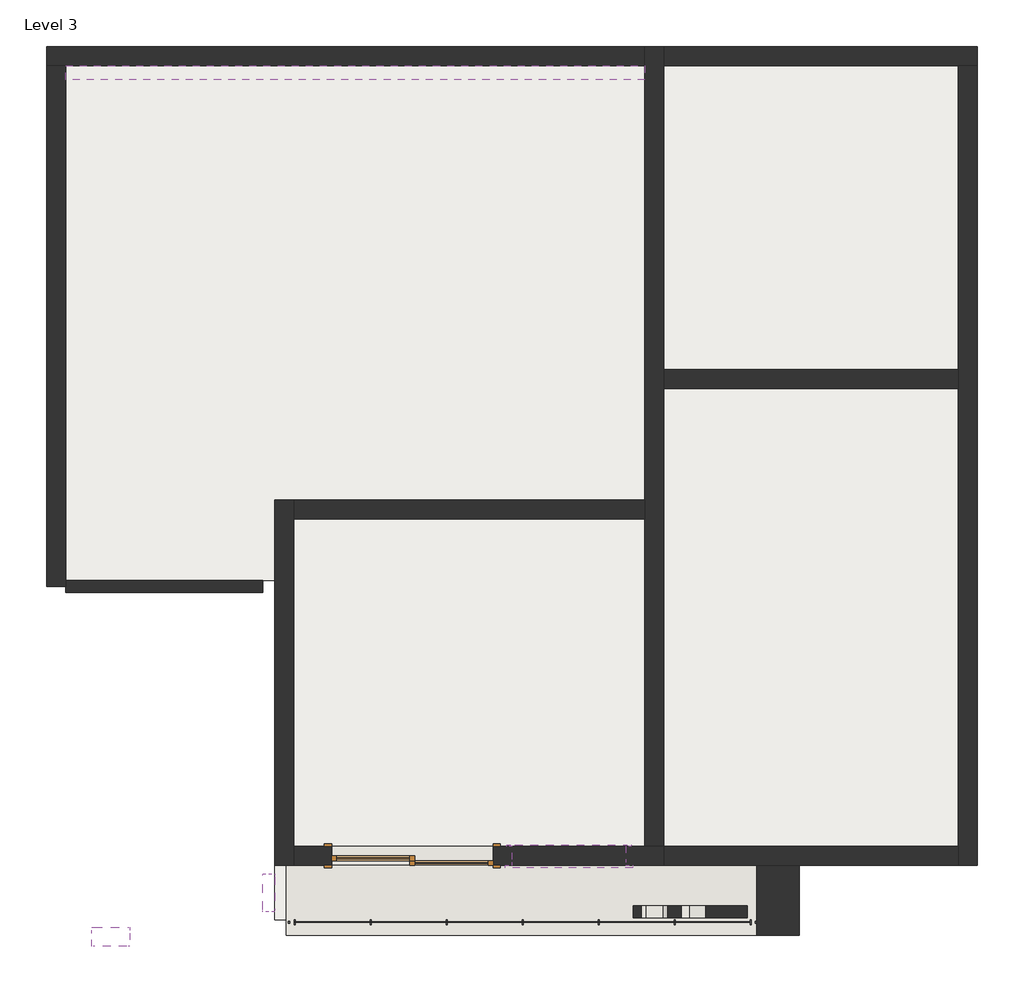
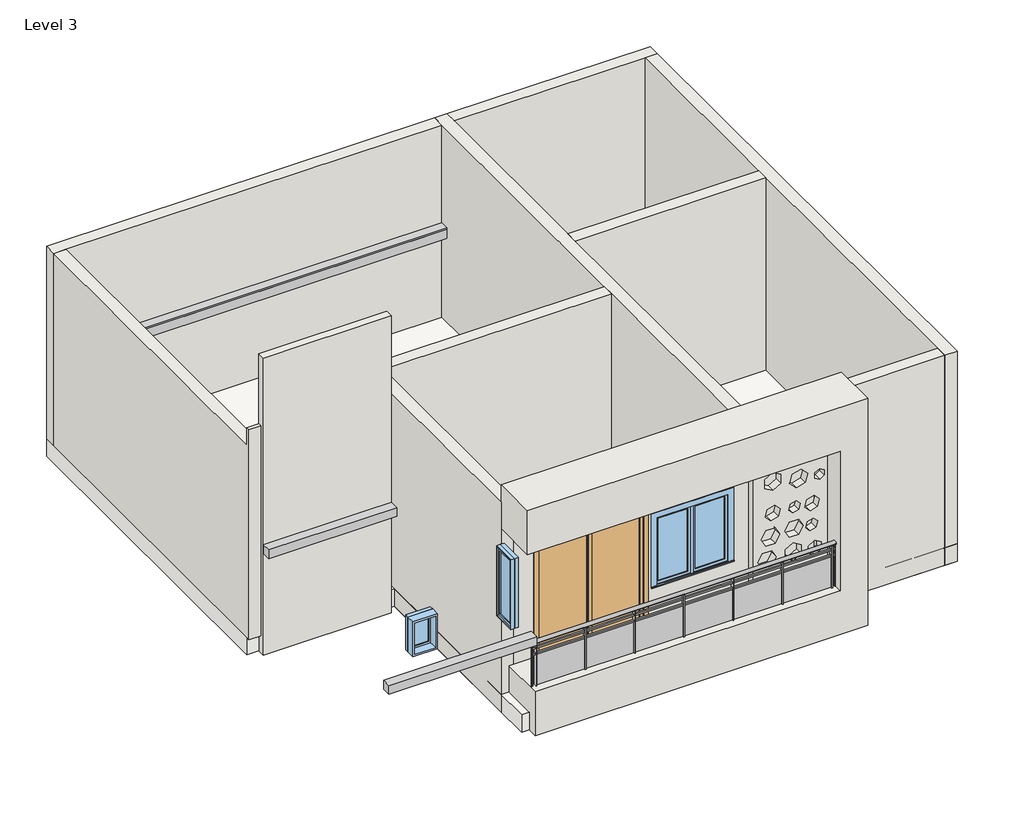
# One storey: 13 walls, 3 windows, 2 proxies, 1 door, 1 railing, 1 roof.
"""IFC4 building model written with IfcOpenShell, lengths in millimetres."""

from ifc_helpers import new_model, si_unit, point, frame, origin, place, context, project, spatial, polyline, ellipse_curve, trimmed, outline, extrude, faceted_brep, transform, mapped, element, save
from ifc_brep_helpers import plane_surface, extruded_surface, advanced_brep
from components import door_076b30e0, walls_1_walls_1_5292a9a1, window_0862ab64, window_085f26e1, window_f83fec05

model = new_model("IFC4")

# Units and contexts
model_context = context("Model", 3, world=origin())
ifc_project = project(units=[si_unit("LENGTHUNIT", "METRE", prefix="MILLI")], contexts=[model_context])

# Site, building, storey
site = spatial("IfcSite", under=ifc_project)
building = spatial("IfcBuilding", under=site)
storey = spatial("IfcBuildingStorey", under=building, Name="Level 3", Elevation=7315.2)

# Proxies
placement = place(None, origin())
element("IfcBuildingElementProxy", 1, Name="Cornice", ObjectType="Cornice", at=placement, inside=storey, context=model_context, shape_type="SweptSolid", body=[
    extrude(outline(polyline([(-5898.9432037, 9807.0548743), (-5898.9432037, 9654.6548743), (-12096.5432037, 9654.6548743), (-12096.5432037, 9807.0548743), (-5898.9432037, 9807.0548743)])), frame((0.0, 0.0, 9093.2), z_axis=(0.0, 0.0, 1.0), x_axis=(1.0, 0.0, 0.0)), (0.0, 0.0, 1.0), 152.4),
    extrude(outline(polyline([(-12299.7432037, 231.2548743), (-12299.7432037, 383.6548743), (-9861.3432037, 383.6548743), (-9861.3432037, 231.2548743), (-12299.7432037, 231.2548743)])), frame((0.0, 0.0, 9093.2), z_axis=(0.0, 0.0, 1.0), x_axis=(1.0, 0.0, 0.0)), (0.0, 0.0, 1.0), 152.4),
    extrude(outline(polyline([(-9988.3432037, 4168.2548743), (-9988.3432037, 4015.8548743), (-12096.5432037, 4015.8548743), (-12096.5432037, 4168.2548743), (-9988.3432037, 4168.2548743)])), frame((0.0, 0.0, 9093.2), z_axis=(0.0, 0.0, 1.0), x_axis=(1.0, 0.0, 0.0)), (0.0, 0.0, 1.0), 152.4),
])
element("IfcBuildingElementProxy", 2, Name="Cornice", ObjectType="Cornice", at=placement, inside=storey, context=model_context, shape_type="SweptSolid", body=[
    extrude(outline(polyline([(-5898.9432037, 9807.0548743), (-5898.9432037, 9654.6548743), (-12096.5432037, 9654.6548743), (-12096.5432037, 9807.0548743), (-5898.9432037, 9807.0548743)])), frame((0.0, 0.0, 9118.6), z_axis=(0.0, 0.0, 1.0), x_axis=(1.0, 0.0, 0.0)), (0.0, 0.0, 1.0), 152.4),
])

# Door
door_shape = door_076b30e0(model_context)
element("IfcDoor", 3, ObjectType="Door-Double-Sliding : 68\" x 80\"", at=placement, inside=storey, context=model_context, shape_type="MappedRepresentation", body=[
    mapped(door_shape, transform((-8388.1432037, 1475.8548743, 7924.8), x_axis=(-1.0, 0.0, 0.0), y_axis=(0.0, -1.0, 0.0), z_axis=(0.0, 0.0, 1.0))),
])

# Railing
element("IfcRailing", 4, ObjectType="Glass Panel - Bottom Fill", at=placement, inside=storey, context=model_context, shape_type="SolidModel", body=[
    advanced_brep(
    [(-9708.9432037, 675.7548743, 8839.2), (-9708.9432037, 599.5548743, 8839.2), (-4705.1432037, 675.7548743, 8839.2), (-4705.1432037, 599.5548743, 8839.2)],
    [
        (0, 1, ellipse_curve(frame((-9708.9432037, 637.6548743, 8839.2), z_axis=(-1.0, 0.0, 0.0), x_axis=(0.0, -1.0, 0.0)), 38.1, 28.575)),
        (1, 0, ellipse_curve(frame((-9708.9432037, 637.6548743, 8839.2), z_axis=(-1.0, 0.0, 0.0), x_axis=(0.0, -1.0, 0.0)), 38.1, 28.575)),
        (2, 3, ellipse_curve(frame((-4705.1432037, 637.6548743, 8839.2), z_axis=(1.0, 0.0, 0.0), x_axis=(0.0, -1.0, 0.0)), 38.1, 28.575)),
        (3, 2, ellipse_curve(frame((-4705.1432037, 637.6548743, 8839.2), z_axis=(1.0, 0.0, 0.0), x_axis=(0.0, -1.0, 0.0)), 38.1, 28.575)),
        (0, 2),
        (3, 1),
    ],
    [
        plane_surface(frame((-9708.9432037, 637.6548743, 8839.2), z_axis=(-1.0, 0.0, 0.0), x_axis=(0.0, 1.0, 0.0))),
        plane_surface(frame((-4705.1432037, 637.6548743, 8839.2), z_axis=(1.0, 0.0, 0.0), x_axis=(0.0, 1.0, 0.0))),
        extruded_surface(trimmed(ellipse_curve(frame((-4705.1432037, 637.6548743, 8839.2), z_axis=(-1.0, 0.0, 0.0), x_axis=(0.0, -1.0, 0.0)), 38.1, 28.575), [point((-4705.1432037, 675.7548743, 8839.2))], [point((-4705.1432037, 599.5548743, 8839.2))], True, "CARTESIAN"), (-5003.8, 0.0, 0.0), 5003.8),
        extruded_surface(trimmed(ellipse_curve(frame((-4705.1432037, 637.6548743, 8839.2), z_axis=(-1.0, 0.0, 0.0), x_axis=(0.0, -1.0, 0.0)), 38.1, 28.575), [point((-4705.1432037, 599.5548743, 8839.2))], [point((-4705.1432037, 675.7548743, 8839.2))], True, "CARTESIAN"), (-5003.8, 0.0, 0.0), 5003.8),
    ],
    [
        (0, [[1, 2]]),
        (1, [[3, 4]]),
        (2, [[-1, 5, -4, 6]]),
        (3, [[-2, -6, -3, -5]]),
    ],
),
    extrude(outline(polyline([(-9708.9432037, 624.9548743), (-9708.9432037, 650.3548743), (-4705.1432037, 650.3548743), (-4705.1432037, 624.9548743), (-9708.9432037, 624.9548743)])), frame((0.0, 0.0, 8724.9), z_axis=(0.0, 0.0, 1.0), x_axis=(1.0, 0.0, 0.0)), (0.0, 0.0, 1.0), 25.4),
    extrude(outline(polyline([(-9708.9432037, 624.9548743), (-9708.9432037, 650.3548743), (-4705.1432037, 650.3548743), (-4705.1432037, 624.9548743), (-9708.9432037, 624.9548743)])), frame((0.0, 0.0, 8623.3), z_axis=(0.0, 0.0, 1.0), x_axis=(1.0, 0.0, 0.0)), (0.0, 0.0, 1.0), 25.4),
    extrude(outline(polyline([(-4774.9932037, 612.2548743), (-4774.9932037, 663.0548743), (-4762.2932037, 663.0548743), (-4762.2932037, 612.2548743), (-4774.9932037, 612.2548743)])), frame((0.0, 0.0, 7924.8), z_axis=(0.0, 0.0, 1.0), x_axis=(1.0, 0.0, 0.0)), (0.0, 0.0, 1.0), 885.6788223),
    extrude(outline(polyline([(-5581.4432037, 644.1900313), (-4768.6432037, 644.1900313), (-4768.6432037, 637.8400313), (-5581.4432037, 637.8400313), (-5581.4432037, 644.1900313)])), frame((0.0, 0.0, 8026.4), z_axis=(0.0, 0.0, 1.0), x_axis=(1.0, 0.0, 0.0)), (0.0, 0.0, 1.0), 596.9),
    extrude(outline(polyline([(-5587.7932037, 612.2548743), (-5587.7932037, 663.0548743), (-5575.0932037, 663.0548743), (-5575.0932037, 612.2548743), (-5587.7932037, 612.2548743)])), frame((0.0, 0.0, 7924.8), z_axis=(0.0, 0.0, 1.0), x_axis=(1.0, 0.0, 0.0)), (0.0, 0.0, 1.0), 885.6788223),
    extrude(outline(polyline([(-6394.2432037, 644.1900313), (-5581.4432037, 644.1900313), (-5581.4432037, 637.8400313), (-6394.2432037, 637.8400313), (-6394.2432037, 644.1900313)])), frame((0.0, 0.0, 8026.4), z_axis=(0.0, 0.0, 1.0), x_axis=(1.0, 0.0, 0.0)), (0.0, 0.0, 1.0), 596.9),
    extrude(outline(polyline([(-6400.5932037, 612.2548743), (-6400.5932037, 663.0548743), (-6387.8932037, 663.0548743), (-6387.8932037, 612.2548743), (-6400.5932037, 612.2548743)])), frame((0.0, 0.0, 7924.8), z_axis=(0.0, 0.0, 1.0), x_axis=(1.0, 0.0, 0.0)), (0.0, 0.0, 1.0), 885.6788223),
    extrude(outline(polyline([(-7207.0432037, 644.1900313), (-6394.2432037, 644.1900313), (-6394.2432037, 637.8400313), (-7207.0432037, 637.8400313), (-7207.0432037, 644.1900313)])), frame((0.0, 0.0, 8026.4), z_axis=(0.0, 0.0, 1.0), x_axis=(1.0, 0.0, 0.0)), (0.0, 0.0, 1.0), 596.9),
    extrude(outline(polyline([(-7213.3932037, 612.2548743), (-7213.3932037, 663.0548743), (-7200.6932037, 663.0548743), (-7200.6932037, 612.2548743), (-7213.3932037, 612.2548743)])), frame((0.0, 0.0, 7924.8), z_axis=(0.0, 0.0, 1.0), x_axis=(1.0, 0.0, 0.0)), (0.0, 0.0, 1.0), 885.6788223),
    extrude(outline(polyline([(-8019.8432037, 644.1900313), (-7207.0432037, 644.1900313), (-7207.0432037, 637.8400313), (-8019.8432037, 637.8400313), (-8019.8432037, 644.1900313)])), frame((0.0, 0.0, 8026.4), z_axis=(0.0, 0.0, 1.0), x_axis=(1.0, 0.0, 0.0)), (0.0, 0.0, 1.0), 596.9),
    extrude(outline(polyline([(-8026.1932037, 612.2548743), (-8026.1932037, 663.0548743), (-8013.4932037, 663.0548743), (-8013.4932037, 612.2548743), (-8026.1932037, 612.2548743)])), frame((0.0, 0.0, 7924.8), z_axis=(0.0, 0.0, 1.0), x_axis=(1.0, 0.0, 0.0)), (0.0, 0.0, 1.0), 885.6788223),
    extrude(outline(polyline([(-8832.6432037, 644.1900313), (-8019.8432037, 644.1900313), (-8019.8432037, 637.8400313), (-8832.6432037, 637.8400313), (-8832.6432037, 644.1900313)])), frame((0.0, 0.0, 8026.4), z_axis=(0.0, 0.0, 1.0), x_axis=(1.0, 0.0, 0.0)), (0.0, 0.0, 1.0), 596.9),
    extrude(outline(polyline([(-8838.9932037, 612.2548743), (-8838.9932037, 663.0548743), (-8826.2932037, 663.0548743), (-8826.2932037, 612.2548743), (-8838.9932037, 612.2548743)])), frame((0.0, 0.0, 7924.8), z_axis=(0.0, 0.0, 1.0), x_axis=(1.0, 0.0, 0.0)), (0.0, 0.0, 1.0), 885.6788223),
    extrude(outline(polyline([(-9645.4432037, 644.1900313), (-8832.6432037, 644.1900313), (-8832.6432037, 637.8400313), (-9645.4432037, 637.8400313), (-9645.4432037, 644.1900313)])), frame((0.0, 0.0, 8026.4), z_axis=(0.0, 0.0, 1.0), x_axis=(1.0, 0.0, 0.0)), (0.0, 0.0, 1.0), 596.9),
    extrude(outline(polyline([(-9651.7932037, 612.2548743), (-9651.7932037, 663.0548743), (-9639.0932037, 663.0548743), (-9639.0932037, 612.2548743), (-9651.7932037, 612.2548743)])), frame((0.0, 0.0, 7924.8), z_axis=(0.0, 0.0, 1.0), x_axis=(1.0, 0.0, 0.0)), (0.0, 0.0, 1.0), 885.6788223),
    extrude(outline(polyline([(-4717.8432037, 628.1298743), (-4717.8432037, 647.1798743), (-4698.7932037, 647.1798743), (-4698.7932037, 628.1298743), (-4717.8432037, 628.1298743)])), frame((0.0, 0.0, 7924.8), z_axis=(0.0, 0.0, 1.0), x_axis=(1.0, 0.0, 0.0)), (0.0, 0.0, 1.0), 885.6788223),
    extrude(outline(polyline([(-9715.2932037, 628.1298743), (-9715.2932037, 647.1798743), (-9696.2432037, 647.1798743), (-9696.2432037, 628.1298743), (-9715.2932037, 628.1298743)])), frame((0.0, 0.0, 7924.8), z_axis=(0.0, 0.0, 1.0), x_axis=(1.0, 0.0, 0.0)), (0.0, 0.0, 1.0), 885.6788223),
])

# Roof
element("IfcRoof", 5, ObjectType="Generic - 12\"", at=placement, inside=storey, context=model_context, shape_type="SweptSolid", body=[
    extrude(outline(polyline([(-12299.7432037, 10010.2548743), (-2342.9432037, 10010.2548743), (-2342.9432037, 1247.2548743), (-4247.9432037, 1247.2548743), (-4247.9432037, 663.0548743), (-9861.3432037, 663.0548743), (-9861.3432037, 1298.0548743), (-9861.3432037, 4295.2548743), (-12299.7432037, 4295.2548743), (-12299.7432037, 10010.2548743)])), frame((0.0, 0.0, 7315.2), z_axis=(0.0, 0.0, 1.0), x_axis=(1.0, 0.0, 0.0)), (0.0, 0.0, 1.0), 304.8),
])

# Walls
element("IfcWall", 6, ObjectType="Generic - 5\"", at=placement, inside=storey, context=model_context, shape_type="Brep", body=[
    faceted_brep([(-9988.3432037, 4295.2548743, 7315.2), (-12096.5432037, 4295.2548743, 7315.2), (-12096.5432037, 4295.2548743, 7620.0), (-12096.5432037, 4295.2548743, 10972.8), (-12096.5432037, 4295.2548743, 11277.6), (-12096.5432037, 4295.2548743, 12496.8), (-9988.3432037, 4295.2548743, 12496.8), (-9988.3432037, 4168.2548743, 7315.2), (-9988.3432037, 4168.2548743, 12496.8), (-12096.5432037, 4168.2548743, 12496.8), (-12096.5432037, 4168.2548743, 7315.2), (-12096.5432037, 4231.7548743, 7315.2)], [[[0, 1, 2, 3, 4, 5, 6]], [[7, 8, 9, 10]], [[1, 0, 7, 10, 11]], [[6, 5, 9, 8]], [[0, 6, 8, 7]], [[1, 11, 10, 9, 5, 4, 3, 2]]]),
])
element("IfcWall", 7, ObjectType="Generic - 5\"", at=placement, inside=storey, context=model_context, shape_type="SweptSolid", body=[
    extrude(outline(polyline([(8068.6361055, -4806.7432037), (10508.7650496, -4806.7432037), (10508.7650496, -6025.9432037), (8068.6361055, -6025.9432037), (8068.6361055, -4806.7432037)]), holes=[polyline([(10140.6755343, -5569.437477), (10064.4755343, -5701.4197485), (10140.6755343, -5833.4020201), (10293.0755343, -5833.4020201), (10369.2755343, -5701.4197485), (10293.0755343, -5569.437477), (10140.6755343, -5569.437477)]), polyline([(10163.9613965, -5130.2790834), (10016.7543006, -5169.7231059), (9977.3102781, -5316.9302018), (10085.0733516, -5424.6932753), (10232.2804475, -5385.2492528), (10271.72447, -5238.0421569), (10163.9613965, -5130.2790834)]), polyline([(9703.2041949, -5578.7471686), (9580.531615, -5611.6171873), (9547.6615962, -5734.2897672), (9637.4641574, -5824.0923285), (9760.1367374, -5791.2223097), (9793.0067561, -5668.5497298), (9703.2041949, -5578.7471686)]), polyline([(9678.1574319, -5247.2726782), (9580.019368, -5273.5686932), (9553.723353, -5371.7067571), (9625.565402, -5443.5488061), (9723.7034659, -5417.2527911), (9749.9994809, -5319.1147272), (9678.1574319, -5247.2726782)]), polyline([(9264.0488124, -5590.7002981), (9132.0665409, -5666.9002981), (9132.0665409, -5819.3002981), (9264.0488124, -5895.5002981), (9396.0310839, -5819.3002981), (9396.0310839, -5666.9002981), (9264.0488124, -5590.7002981)]), polyline([(9279.67242, -5201.6464153), (9147.6901485, -5277.8464153), (9147.6901485, -5430.2464153), (9279.67242, -5506.4464153), (9411.6546915, -5430.2464153), (9411.6546915, -5277.8464153), (9279.67242, -5201.6464153)]), polyline([(9272.6391638, -4966.188489), (9174.5010999, -4992.484504), (9148.2050849, -5090.6225679), (9220.0471339, -5162.4646169), (9318.1851978, -5136.1686019), (9344.4812128, -5038.030538), (9272.6391638, -4966.188489)]), polyline([(9646.9071324, -4934.22274), (9524.2345525, -4967.0927588), (9491.3645338, -5089.7653387), (9581.167095, -5179.5678999), (9703.8396749, -5146.6978812), (9736.7096937, -5024.0253012), (9646.9071324, -4934.22274)]), polyline([(10035.431483, -4853.8956856), (9990.3878062, -4931.9136222), (10035.431483, -5009.9315589), (10125.5188364, -5009.9315589), (10170.5625131, -4931.9136222), (10125.5188364, -4853.8956856), (10035.431483, -4853.8956856)]), polyline([(8887.3926853, -5644.9432037), (8755.4104138, -5721.1432037), (8755.4104138, -5873.5432037), (8887.3926853, -5949.7432037), (9019.3749569, -5873.5432037), (9019.3749569, -5721.1432037), (8887.3926853, -5644.9432037)]), polyline([(8801.9964308, -5235.9460501), (8725.7964308, -5367.9283217), (8801.9964308, -5499.9105932), (8954.3964308, -5499.9105932), (9030.5964308, -5367.9283217), (8954.3964308, -5235.9460501), (8801.9964308, -5235.9460501)]), polyline([(8761.231321, -4901.3742658), (8697.731321, -5011.3594921), (8761.231321, -5121.3447183), (8888.231321, -5121.3447183), (8951.731321, -5011.3594921), (8888.231321, -4901.3742658), (8761.231321, -4901.3742658)]), polyline([(8450.6104138, -5618.3643314), (8295.6101636, -5707.8537676), (8295.6101636, -5886.8326399), (8450.6104138, -5976.3220761), (8605.610664, -5886.8326399), (8605.610664, -5707.8537676), (8450.6104138, -5618.3643314)]), polyline([(8468.3460703, -5203.5482833), (8295.6101636, -5249.83273), (8249.3257169, -5422.5686367), (8375.7771769, -5549.0200966), (8548.5130835, -5502.7356499), (8594.7975302, -5329.9997433), (8468.3460703, -5203.5482833)]), polyline([(8389.7874753, -4898.3582178), (8278.2141342, -4928.2542045), (8248.3181476, -5039.8275455), (8329.995502, -5121.5048999), (8441.5688431, -5091.6089133), (8471.4648297, -4980.0355722), (8389.7874753, -4898.3582178)])]), frame((0.0, 688.4548476, 0.0), z_axis=(0.0, 1.0, 0.0), x_axis=(0.0, 0.0, 1.0)), (0.0, 0.0, 1.0), 127.0),
])
element("IfcWall", 8, ObjectType="Generic - 8\"", at=placement, inside=storey, context=model_context, shape_type="Brep", body=[
    faceted_brep([(-9861.3432037, 5158.8548743, 7315.2), (-9861.3432037, 1247.2548743, 7315.2), (-9861.3432037, 1247.2548743, 10972.8), (-9861.3432037, 1298.0548743, 10972.8), (-9861.3432037, 4295.2548743, 10972.8), (-9861.3432037, 5158.8548743, 10972.8), (-9658.1432037, 5158.8548743, 7315.2), (-9658.1432037, 5158.8548743, 10972.8), (-9658.1432037, 4955.6548743, 10972.8), (-9658.1432037, 1450.4548743, 10972.8), (-9658.1432037, 1247.2548743, 10972.8), (-9658.1432037, 1247.2548743, 7315.2), (-9658.1432037, 1450.4548743, 7315.2), (-9658.1432037, 4955.6548743, 7315.2)], [[[0, 1, 2, 3, 4, 5]], [[6, 7, 8, 9, 10, 11, 12, 13]], [[1, 0, 6, 13, 12, 11]], [[2, 1, 11, 10]], [[0, 5, 7, 6]], [[5, 4, 3, 2, 10, 9, 8, 7]]]),
])
element("IfcWall", 9, ObjectType="Generic - 8\"", at=placement, inside=storey, context=model_context, shape_type="Brep", body=[
    faceted_brep([(-9658.1432037, 1247.2548743, 7315.2), (-5695.7432037, 1247.2548743, 7315.2), (-5695.7432037, 1247.2548743, 10972.8), (-9658.1432037, 1247.2548743, 10972.8), (-7524.5432037, 1247.2548743, 9956.8), (-7524.5432037, 1247.2548743, 7924.8), (-9251.7432037, 1247.2548743, 7924.8), (-9251.7432037, 1247.2548743, 9956.8), (-7321.3432037, 1247.2548743, 9833.9107901), (-6102.1432037, 1247.2548743, 9833.9107901), (-6102.1432037, 1247.2548743, 8614.7107901), (-7321.3432037, 1247.2548743, 8614.7107901), (-9658.1432037, 1450.4548743, 7315.2), (-9658.1432037, 1450.4548743, 10972.8), (-5898.9432037, 1450.4548743, 10972.8), (-5695.7432037, 1450.4548743, 10972.8), (-5695.7432037, 1450.4548743, 7315.2), (-5898.9432037, 1450.4548743, 7315.2), (-7524.5432037, 1450.4548743, 9956.8), (-9251.7432037, 1450.4548743, 9956.8), (-9251.7432037, 1450.4548743, 7924.8), (-7524.5432037, 1450.4548743, 7924.8), (-7321.3432037, 1450.4548743, 9833.9107901), (-7321.3432037, 1450.4548743, 8614.7107901), (-6102.1432037, 1450.4548743, 8614.7107901), (-6102.1432037, 1450.4548743, 9833.9107901)], [[[0, 1, 2, 3], [4, 5, 6, 7], [8, 9, 10, 11]], [[12, 13, 14, 15, 16, 17], [18, 19, 20, 21], [22, 23, 24, 25]], [[1, 0, 12, 17, 16]], [[0, 3, 13, 12]], [[2, 1, 16, 15]], [[3, 2, 15, 14, 13]], [[5, 4, 18, 21]], [[6, 5, 21, 20]], [[7, 6, 20, 19]], [[4, 7, 19, 18]], [[23, 22, 8, 11]], [[24, 23, 11, 10]], [[25, 24, 10, 9]], [[22, 25, 9, 8]]]),
])
element("IfcWall", 10, ObjectType="Generic - 8\"", at=placement, inside=storey, context=model_context, shape_type="Brep", body=[
    faceted_brep([(-5695.7432037, 1450.4548743, 7315.2), (-5695.7432037, 6352.6548743, 7315.2), (-5695.7432037, 6555.8548743, 7315.2), (-5695.7432037, 9807.0548743, 7315.2), (-5695.7432037, 10010.2548743, 7315.2), (-5695.7432037, 10010.2548743, 10972.8), (-5695.7432037, 9807.0548743, 10972.8), (-5695.7432037, 6555.8548743, 10972.8), (-5695.7432037, 6352.6548743, 10972.8), (-5695.7432037, 5362.0548743, 10972.8), (-5695.7432037, 1450.4548743, 10972.8), (-5898.9432037, 1450.4548743, 7315.2), (-5898.9432037, 1450.4548743, 10972.8), (-5898.9432037, 4955.6548743, 10972.8), (-5898.9432037, 5158.8548743, 10972.8), (-5898.9432037, 5362.0548743, 10972.8), (-5898.9432037, 9807.0548743, 10972.8), (-5898.9432037, 10010.2548743, 10972.8), (-5898.9432037, 10010.2548743, 7620.0), (-5898.9432037, 10010.2548743, 7315.2), (-5898.9432037, 5158.8548743, 7315.2), (-5898.9432037, 4955.6548743, 7315.2)], [[[0, 1, 2, 3, 4, 5, 6, 7, 8, 9, 10]], [[11, 12, 13, 14, 15, 16, 17, 18, 19, 20, 21]], [[4, 3, 2, 1, 0, 11, 21, 20, 19]], [[0, 10, 12, 11]], [[10, 9, 8, 7, 6, 5, 17, 16, 15, 14, 13, 12]], [[4, 19, 18, 17, 5]]]),
])
element("IfcWall", 11, ObjectType="Generic - 8\"", at=placement, inside=storey, context=model_context, shape_type="SweptSolid", body=[
    extrude(outline(polyline([(-2546.1432037, 6352.6548743), (-5695.7432037, 6352.6548743), (-5695.7432037, 6555.8548743), (-2546.1432037, 6555.8548743), (-2546.1432037, 6352.6548743)])), frame((0.0, 0.0, 7315.2), z_axis=(0.0, 0.0, 1.0), x_axis=(1.0, 0.0, 0.0)), (0.0, 0.0, 1.0), 3657.6),
])
element("IfcWall", 12, ObjectType="Generic - 8\"", at=placement, inside=storey, context=model_context, shape_type="Brep", body=[
    faceted_brep([(-2546.1432037, 9807.0548743, 7315.2), (-2546.1432037, 6555.8548743, 7315.2), (-2546.1432037, 6352.6548743, 7315.2), (-2546.1432037, 1450.4548743, 7315.2), (-2546.1432037, 1247.2548743, 7315.2), (-2546.1432037, 1247.2548743, 10972.8), (-2546.1432037, 1450.4548743, 10972.8), (-2546.1432037, 6352.6548743, 10972.8), (-2546.1432037, 6555.8548743, 10972.8), (-2546.1432037, 9807.0548743, 10972.8), (-2342.9432037, 9807.0548743, 7315.2), (-2342.9432037, 9807.0548743, 10972.8), (-2342.9432037, 1247.2548743, 10972.8), (-2342.9432037, 1247.2548743, 7315.2)], [[[0, 1, 2, 3, 4, 5, 6, 7, 8, 9]], [[10, 11, 12, 13]], [[4, 3, 2, 1, 0, 10, 13]], [[5, 4, 13, 12]], [[0, 9, 11, 10]], [[9, 8, 7, 6, 5, 12, 11]]]),
])
element("IfcWall", 13, ObjectType="Generic - 8\"", at=placement, inside=storey, context=model_context, shape_type="Brep", body=[
    faceted_brep([(-5695.7432037, 1247.2548743, 7315.2), (-2546.1432037, 1247.2548743, 7315.2), (-2546.1432037, 1247.2548743, 10972.8), (-4247.9432037, 1247.2548743, 10972.8), (-5695.7432037, 1247.2548743, 10972.8), (-5695.7432037, 1450.4548743, 7315.2), (-5695.7432037, 1450.4548743, 10972.8), (-2546.1432037, 1450.4548743, 10972.8), (-2546.1432037, 1450.4548743, 7315.2)], [[[0, 1, 2, 3, 4]], [[5, 6, 7, 8]], [[1, 0, 5, 8]], [[0, 4, 6, 5]], [[2, 1, 8, 7]], [[4, 3, 2, 7, 6]]]),
])
element("IfcWall", 14, ObjectType="Generic - 8\"", at=placement, inside=storey, context=model_context, shape_type="SweptSolid", body=[
    extrude(outline(polyline([(-5898.9432037, 4955.6548743), (-9658.1432037, 4955.6548743), (-9658.1432037, 5158.8548743), (-5898.9432037, 5158.8548743), (-5898.9432037, 4955.6548743)])), frame((0.0, 0.0, 7315.2), z_axis=(0.0, 0.0, 1.0), x_axis=(1.0, 0.0, 0.0)), (0.0, 0.0, 1.0), 3657.6),
])
element("IfcWall", 15, ObjectType="Generic - 8\"", at=placement, inside=storey, context=model_context, shape_type="Brep", body=[
    faceted_brep([(-5695.7432037, 9807.0548743, 10972.8), (-5695.7432037, 9807.0548743, 7315.2), (-2546.1432037, 9807.0548743, 7315.2), (-2342.9432037, 9807.0548743, 7315.2), (-2342.9432037, 9807.0548743, 10972.8), (-2546.1432037, 9807.0548743, 10972.8), (-5695.7432037, 10010.2548743, 7315.2), (-5695.7432037, 10010.2548743, 10972.8), (-2342.9432037, 10010.2548743, 10972.8), (-2342.9432037, 10010.2548743, 7315.2), (-5695.7432037, 9832.4548743, 10972.8)], [[[0, 1, 2, 3, 4, 5]], [[6, 7, 8, 9]], [[3, 2, 1, 6, 9]], [[4, 3, 9, 8]], [[0, 5, 4, 8, 7, 10]], [[0, 10, 7, 6, 1]]]),
])
element("IfcWall", 16, ObjectType="Generic - 8\"", at=placement, inside=storey, context=model_context, shape_type="Brep", body=[
    faceted_brep([(-5898.9432037, 10010.2548743, 10972.8), (-5898.9432037, 10010.2548743, 7620.0), (-12299.7432037, 10010.2548743, 7620.0), (-12299.7432037, 10010.2548743, 10972.8), (-5898.9432037, 9807.0548743, 7620.0), (-5898.9432037, 9807.0548743, 10972.8), (-12096.5432037, 9807.0548743, 10972.8), (-12299.7432037, 9807.0548743, 10972.8), (-12299.7432037, 9807.0548743, 7620.0), (-12096.5432037, 9807.0548743, 7620.0)], [[[0, 1, 2, 3]], [[4, 5, 6, 7, 8, 9]], [[2, 1, 4, 9, 8]], [[3, 2, 8, 7]], [[0, 3, 7, 6, 5]], [[0, 5, 4, 1]]]),
])
element("IfcWall", 17, ObjectType="Generic - 8\"", at=placement, inside=storey, context=model_context, shape_type="Brep", body=[
    faceted_brep([(-12299.7432037, 9807.0548743, 7620.0), (-12299.7432037, 4295.2548743, 7620.0), (-12299.7432037, 4231.7548743, 7620.0), (-12299.7432037, 4231.7548743, 11277.6), (-12299.7432037, 4295.2548743, 11277.6), (-12299.7432037, 4295.2548743, 10972.8), (-12299.7432037, 9807.0548743, 10972.8), (-12096.5432037, 4231.7548743, 7620.0), (-12096.5432037, 4295.2548743, 7620.0), (-12096.5432037, 9807.0548743, 7620.0), (-12096.5432037, 9807.0548743, 9093.2), (-12096.5432037, 9807.0548743, 9245.6), (-12096.5432037, 9807.0548743, 10972.8), (-12096.5432037, 4295.2548743, 10972.8), (-12096.5432037, 4295.2548743, 11277.6), (-12096.5432037, 4231.7548743, 11277.6)], [[[0, 1, 2, 3, 4, 5, 6]], [[7, 8, 9, 10, 11, 12, 13, 14, 15]], [[2, 1, 0, 9, 8, 7]], [[3, 2, 7, 15]], [[0, 6, 12, 11, 10, 9]], [[3, 15, 14, 4]], [[12, 6, 5, 13]], [[4, 14, 13, 5]]]),
])
walls_1_walls_1_shape = walls_1_walls_1_5292a9a1(model_context)
element("IfcWall", 18, ObjectType="Walls 1 : Walls 1", at=placement, inside=storey, context=model_context, shape_type="MappedRepresentation", body=[
    mapped(walls_1_walls_1_shape, transform((0.0, 0.0, 0.0), x_axis=(1.0, 0.0, 0.0), y_axis=(0.0, 1.0, 0.0), z_axis=(0.0, 0.0, 1.0))),
])

# Windows
window_shape = window_0862ab64(model_context)
element("IfcWindow", 19, ObjectType="Casement Dbl with Trim : 48\" x 48\"", at=placement, inside=storey, context=model_context, shape_type="MappedRepresentation", body=[
    mapped(window_shape, transform((-6711.7432037, 1367.9048743, 7700.3107901), x_axis=(-1.0, 0.0, 0.0), y_axis=(0.0, -1.0, 0.0), z_axis=(0.0, 0.0, 1.0))),
])
window_2_shape = window_085f26e1(model_context)
element("IfcWindow", 20, ObjectType="Fixed : 16\" x 24\"", at=placement, inside=storey, context=model_context, shape_type="MappedRepresentation", body=[
    mapped(window_2_shape, transform((-11575.8432037, 485.2548743, 8571.2555904), x_axis=(1.0, 0.0, 0.0), y_axis=(0.0, 1.0, 0.0), z_axis=(0.0, 0.0, 1.0))),
])
window_3_shape = window_f83fec05(model_context)
element("IfcWindow", 21, ObjectType="Fixed : 16\" x 48\"", at=placement, inside=storey, context=model_context, shape_type="MappedRepresentation", body=[
    mapped(window_3_shape, transform((-9924.8432037, 993.2548743, 8180.6841054), x_axis=(0.0, 1.0, 0.0), y_axis=(-1.0, 0.0, 0.0), z_axis=(0.0, 0.0, 1.0))),
])

save(model, "model.ifc")

# Revit data of these elements
# Type "Door-Double-Sliding : 68\" x 80\""
#   Type Mark = "8"
#   Construction Type Id = "opn-d45"
#   Assembly Code = "C1020"
#   Analytic Construction = "Wood frame, double glass door "
#   Thickness = 0' - 2"
#   Thermal Resistance (R) = 1.8150 (h·ft²·°F)/BTU
#   Heat Transfer Coefficient (U) = 0.5510 BTU/(h·ft²·°F)
#   Height = 6' - 8"
#   Rail Width = 0' - 2"
#   Stiles = 0' - 2"
#   Trim Projection Ext = 0' - 1"
#   Trim Projection Int = 0' - 1"
#   Trim Width = 0' - 3"
#   Width = 5' - 8"
#   Define Thermal Properties by = 1
#   Glazing = Glass
#   Panel Material = Wood - Birch - Solid Stained Light Low Gloss
#   Trim Material = Paint - Sienna
#   Visual Light Transmittance = 0
#   Solar Heat Gain Coefficient = 0
#   Function = (empty or 0)
#   Wall Closure = (empty or 0)
# Type "Glass Panel - Bottom Fill"
#   Assembly Code = "C2010400"
#   built-in parameter 1008612 = 0.0416667 (stored number, unit not read)
#   built-in parameter 1008611 = 0.0416667 (stored number, unit not read)
#   built-in parameter 1008609 = 0.333333 (stored number, unit not read)
#   built-in parameter 1008604 = 0.166667 (stored number, unit not read)
#   built-in parameter 1008603 = 0.166667 (stored number, unit not read)
#   Railing Height = 3' - 0"
#   built-in parameter 1008630 = 2
#   built-in parameter 1008610 = 2
#   built-in parameter 1008618 = Baluster - Square : 3/4"
# Type "Generic - 12\""
#   Assembly Code = "B1020"
#   Layers, outside or top first: 1' - 0" no material (function 1)
# Type "Generic - 5\""
#   Assembly Code = "B2010"
#   Layers, outside or top first: 0' - 5" no material (function 1)
# Type "Generic - 8\""
#   Assembly Code = "B2010"
#   Layers, outside or top first: 0' - 8" no material (function 1)
# Type "Casement Dbl with Trim : 48\" x 48\""
#   Type Mark = "13"
#   Construction Type Id = "GSP4R"
#   Assembly Code = "B2020100"
#   Analytic Construction = "1/8 in Pilkington single glazing"
#   Visual Light Transmittance = 0.9
#   Thermal Resistance (R) = 1.53941 (h·ft²·°F)/BTU
#   Solar Heat Gain Coefficient = 0.78
#   Heat Transfer Coefficient (U) = 0.6496 BTU/(h·ft²·°F)
#   Height = 4' - 0"
#   Default Sill Height = 3' - 0"
#   Trim Projection - Ext. = 0' - 0 1/2"
#   Trim Projection - Int. = 0' - 0 3/4"
#   Trim Width - Exterior = 0' - 3 1/2"
#   Trim Width - Interior = 0' - 3 1/2"
#   Width = 4' - 0"
#   Window Inset = 0' - 0 3/4"
#   Define Thermal Properties by = 1
#   Glass Pane Material = Glass
#   Sash Material = Sash
#   Trim Exterior Material = Trim
#   Trim Interior Material = Trim
#   Wall Closure = (empty or 0)
# Type "Fixed : 16\" x 24\""
#   Type Mark = "4"
#   Construction Type Id = "GSP4R"
#   Assembly Code = "B2020100"
#   Analytic Construction = "1/8 in Pilkington single glazing"
#   Visual Light Transmittance = 0.9
#   Solar Heat Gain Coefficient = 0.78
#   Heat Transfer Coefficient (U) = 0.6496 BTU/(h·ft²·°F)
#   Height = 2' - 0"
#   Default Sill Height = 3' - 0"
#   Width = 1' - 4"
#   Window Inset = 0' - 0 3/4"
#   Define Thermal Properties by = 1
#   Glass Pane Material = Glass
#   Sash Material = Sash
#   Wall Closure = (empty or 0)
# Type "Fixed : 16\" x 48\""
#   Type Mark = "5"
#   Construction Type Id = "GSP4R"
#   Assembly Code = "B2020100"
#   Analytic Construction = "1/8 in Pilkington single glazing"
#   Visual Light Transmittance = 0.9
#   Solar Heat Gain Coefficient = 0.78
#   Heat Transfer Coefficient (U) = 0.6496 BTU/(h·ft²·°F)
#   Height = 4' - 0"
#   Default Sill Height = 3' - 0"
#   Width = 1' - 4"
#   Window Inset = 0' - 0 3/4"
#   Define Thermal Properties by = 1
#   Glass Pane Material = Glass
#   Sash Material = Sash
#   Wall Closure = (empty or 0)
# Elements 1, 2 (IfcBuildingElementProxy, "Cornice")
#   Phase Created = New Construction
#   Materials on its faces: "Default Wall"
# Element 3 (IfcDoor, "Door-Double-Sliding : 68\" x 80\"")
#   Phase Created = New Construction
#   Materials on its faces: "Paint - Sienna", "Wood - Birch - Solid Stained Light Low Gloss", "Glass"
# Element 4 (IfcRailing, "Glass Panel - Bottom Fill")
#   built-in parameter 1008621 = 2 (stored number, unit not read)
#   Phase Created = New Construction
#   Materials on its faces: "Glass"
# Element 5 (IfcRoof, "Generic - 12\"")
#   built-in parameter 1001705 = 25 (stored number, unit not read)
#   built-in parameter 1001710 = 33615
#   Phase Created = New Construction
#   Materials on its faces: "Default Roof"
# Element 6 (IfcWall, "Generic - 5\"")
#   Top Offset = 5' - 0"
#   Base Offset = 0' - 0"
#   wall height = 17' - 0"
#   Phase Created = New Construction
#   Base Constraint = Level 3
#   Top Constraint = Level 4
#   Materials on its faces: "Default Wall"
# Element 7 (IfcWall, "Generic - 5\"")
#   built-in parameter 1001111 = 2' - 5.66284"
#   Top Offset = -1' - 6.26909"
#   Base Offset = 2' - 5.66284"
#   wall height = 8' - 0.06807"
#   Phase Created = New Construction
#   Base Constraint = Level 3
#   Top Constraint = Level 4
#   Materials on its faces: "Default Wall"
# Elements 8, 9, 10, 11, 12, 13, 14, 15 (IfcWall, "Generic - 8\"")
#   Top Offset = 0' - 0"
#   Base Offset = 0' - 0"
#   Unconnected Height = 12' - 0"
#   wall height = 12' - 0"
#   Phase Created = New Construction
#   Base Constraint = Level 3
#   Materials on its faces: "Default Wall"
# Elements 16, 17 (IfcWall, "Generic - 8\"")
#   built-in parameter 1001111 = 1' - 0"
#   Top Offset = 0' - 0"
#   Base Offset = 1' - 0"
#   Unconnected Height = 12' - 0"
#   wall height = 12' - 0"
#   Phase Created = New Construction
#   Base Constraint = Level 3
#   Materials on its faces: "Default Wall"
# Element 18 (IfcWall, "Walls 1 : Walls 1")
#   Phase Created = New Construction
#   Materials on its faces: "Default Wall"
# Element 19 (IfcWindow, "Casement Dbl with Trim : 48\" x 48\"")
#   Mark = "2"
#   Phase Created = New Construction
#   Materials on its faces: "Sash", "Trim", "Glass"
# Element 20 (IfcWindow, "Fixed : 16\" x 24\"")
#   Mark = "6"
#   Phase Created = New Construction
#   Materials on its faces: "Sash", "Glass"
# Element 21 (IfcWindow, "Fixed : 16\" x 48\"")
#   Mark = "9"
#   Phase Created = New Construction
#   Materials on its faces: "Sash", "Glass"
# Materials
#   "Glass": class "Glass", colour RGB 0 128 192, transparency 0.75, Description = "Soda Lime Glass", Cost = 0
#   "Wood - Birch - Solid Stained Light Low Gloss": class "Wood", colour RGB 210 159 95, transparency 0, Cost = 0
#   "Paint - Sienna": colour RGB 118 70 51, transparency 0, Cost = 0
#   "Sash": class "Wood", colour RGB 224 178 126, transparency 0
#   "Trim": class "Wood", colour RGB 224 178 126, transparency 0
#   "Default Wall": colour RGB 128 128 128, transparency 0
#   "Default Roof": colour RGB 88 101 114, transparency 0
